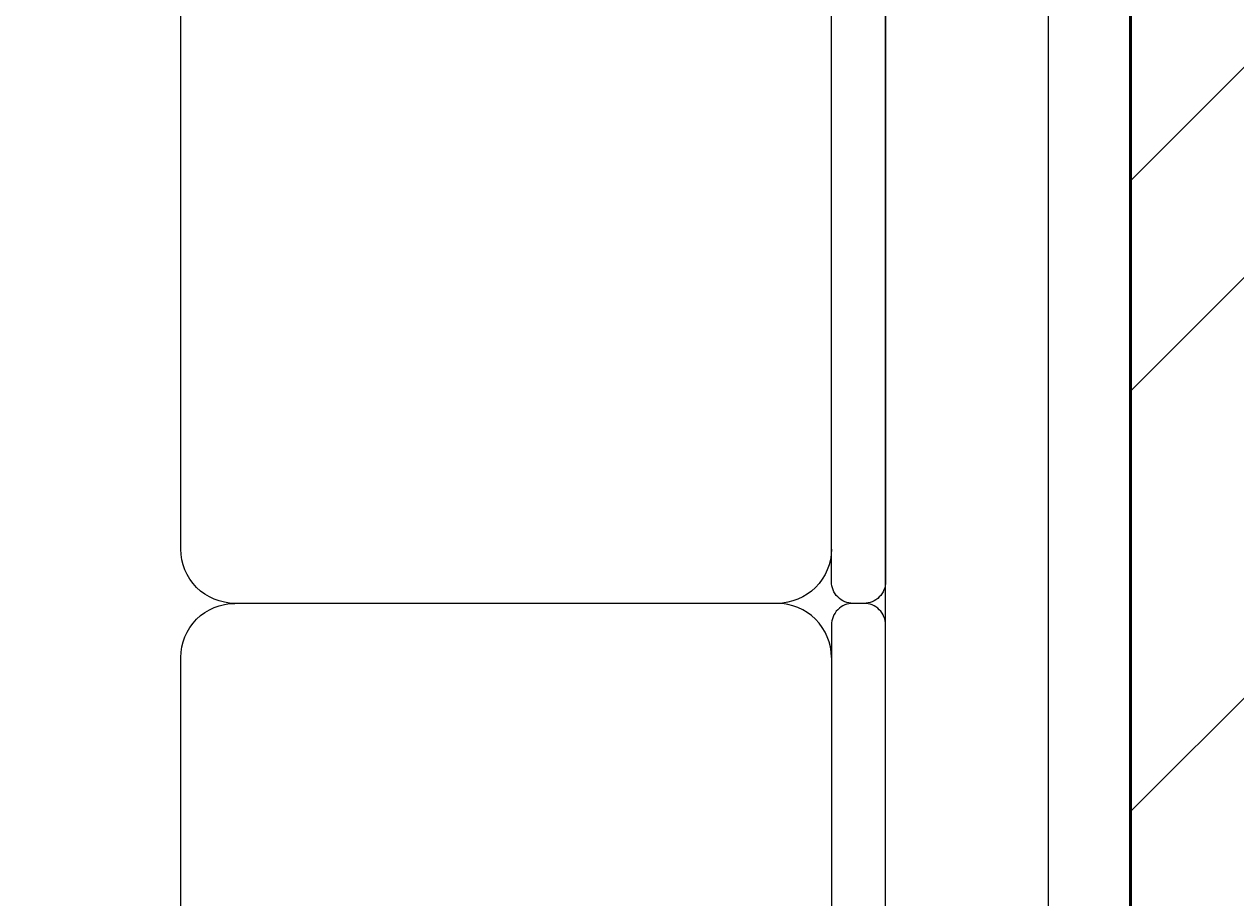
# Model space of a CAD drawing. Units: inches. Extents: x 963 to 2075, y 289 to 2657.
# Tile 23 of 98: x 1485 to 1511, y 1763 to 1781. Entities that reach past the tile are written whole.
import ezdxf

# ---------------------------------------------------------------- set-up
doc = ezdxf.new("R2010")
doc.units = ezdxf.units.IN
for name, color, linetype, lineweight in [('A-ANNO-DIMS', 2, 'Continuous', 18), ('A-FURN', 8, 'Continuous', 18), ('A-WALL', 7, 'Continuous', 50), ('A-WALL-PATT', 8, 'Continuous', 13)]:
    doc.layers.add(name, color=color, linetype=linetype, lineweight=lineweight)
doc.styles.get("Standard").update_dxf_attribs({"font": 'arial.ttf'})
doc.dimstyles.get("Standard").update_dxf_attribs({"dimtxt": 0.18, "dimasz": 0.18, "dimexe": 0.18, "dimexo": 0.0625, "dimgap": 0.09, "dimtad": 0, "dimtih": 1, "dimtoh": 1, "dimdec": 4, "dimzin": 0, "dimdsep": 46, "dimtxsty": 'Standard', "dimcen": 0.09, "dimadec": 0, "dimazin": 0, "dimtfac": 1, "dimtdec": 4, "dimtofl": 0, "dimtmove": 0, "dimatfit": 3, "dimfxl": 1, "dimtolj": 1, "dimtzin": 0, "dimarcsym": 0})

# ---------------------------------------------------------------- blocks, each defined once
blk = doc.blocks.new('SOFA-3SEAT')
at = {"ltscale": 0.03}
blk.add_lwpolyline([(2.442, 16.426, -0.414214), (0.124, 18.743), (0.124, 32.649, -0.414214), (1.283, 33.808, -0.414214), (0.124, 34.967), (0.124, 46.555, -0.414214), (1.283, 47.713, -0.414214), (0.124, 48.872), (0.124, 62.778, -0.414214), (2.442, 65.095), (16.347, 65.095, -0.414214), (18.665, 62.778), (18.665, 18.743, -0.414214), (16.347, 16.426)], format="xyb", close=True, dxfattribs=at)
blk.add_lwpolyline([(15.189, 24.268), (15.189, 51.011)])
blk.add_lwpolyline([(15.189, 47.25), (15.189, 34.271, -0.414214), (14.725, 33.808), (14.493, 33.808, -0.414214), (14.03, 34.271), (14.03, 47.25, -0.414214), (14.493, 47.713), (14.725, 47.713, -0.414214)], format="xyb", close=True)
for points in [[(14.03, 34.967, -0.414214), (12.871, 33.808)], [(14.03, 32.649, 0.414214), (12.871, 33.808), (1.283, 33.808, 0.414214)], [(15.189, 24.268), (15.189, 33.344, 0.414214), (14.725, 33.808), (14.493, 33.808, 0.414214), (14.03, 33.344), (14.03, 25.435, 0.414214)]]:
    blk.add_lwpolyline(points, format="xyb")
blk = doc.blocks.new('*D28')
at = {"layer": 'A-ANNO-DIMS', "color": 0, "lineweight": -2, "transparency": 16777216}
for p, q in [((1506.727, 1816.319), (1519.012, 1816.319)), ((1518.832, 1816.139), (1518.832, 1775.944)), ((1518.832, 1735.382), (1518.832, 1775.577)), ((1506.727, 1735.202), (1519.012, 1735.202))]:
    blk.add_line(p, q, dxfattribs=at)
at = {"layer": 'A-ANNO-DIMS', "color": 0, "transparency": 16777216}
for points in [[(1518.802, 1816.139), (1518.862, 1816.139), (1518.832, 1816.319)], [(1518.802, 1735.382), (1518.862, 1735.382), (1518.832, 1735.202)]]:
    blk.add_solid(points, dxfattribs=at)
at = {"layer": 'Defpoints', "color": 0, "transparency": 16777216}
for p in [(1506.665, 1816.319), (1518.832, 1816.319), (1506.665, 1735.202)]:
    blk.add_point(p, dxfattribs=at)
at = {"layer": 'A-ANNO-DIMS', "color": 0, "transparency": 16777216, "insert": (1518.832, 1775.761), "char_height": 0.18, "attachment_point": 5}
blk.add_mtext('\\A1;3-SEAT SOFA 81 TYP.', dxfattribs=at)

msp = doc.modelspace()

# ---------------------------------------------------------------- hatches: boundary and pattern name
at = {"layer": 'A-WALL-PATT'}
h = msp.add_hatch(dxfattribs=at)
h.set_pattern_fill('ANSI32', color=256)
h.paths.add_polyline_path([(1473.609, 2163.068), (1473.609, 2165.318), (1376.422, 2165.318), (1376.422, 2227.983), (1371.922, 2227.983), (1371.922, 2214.818), (1368.405, 2214.818), (1368.405, 2210.318), (1371.922, 2210.318), (1371.922, 2160.818), (1395.922, 2160.818), (1395.922, 2090.318), (1217.345, 2090.318), (1217.345, 2085.818), (1395.922, 2085.818), (1458.922, 2085.818), (1458.922, 2108.318), (1454.422, 2108.318), (1454.422, 2090.318), (1400.422, 2090.318), (1400.422, 2160.818), (1473.609, 2160.818)])
h.paths.add_polyline_path([(1649.422, 2210.318), (1653.225, 2210.318), (1653.225, 2214.818), (1649.422, 2214.818), (1649.422, 2227.983), (1644.922, 2227.983), (1644.922, 2165.318), (1550.099, 2165.318), (1550.099, 2160.818), (1620.922, 2160.818), (1620.922, 2112.818), (1555.446, 2112.818), (1555.446, 2108.318), (1584.327, 2108.318), (1584.327, 2084.916), (1588.827, 2084.916), (1588.827, 2108.318), (1625.422, 2108.318), (1667.951, 2108.318), (1667.951, 2022.667), (1588.827, 2022.667), (1588.827, 2047.408), (1584.327, 2047.408), (1584.327, 1996.003), (1588.827, 1996.003), (1588.827, 2018.318), (1667.951, 2018.167), (1667.951, 1928.318), (1625.422, 1928.318), (1625.422, 1923.818), (1672.451, 1923.818), (1672.451, 1928.318), (1672.451, 1946.663), (1785.446, 1946.663), (1785.446, 1951.163), (1743.034, 1951.163), (1743.034, 2017.922), (1841.422, 2017.922), (1841.422, 2014.775), (1845.922, 2014.775), (1845.922, 2017.922), (1905.922, 2017.922), (1905.922, 1987.511), (1910.422, 1987.511), (1910.422, 2022.422), (1910.422, 2068.517), (1905.922, 2068.517), (1905.922, 2022.422), (1845.922, 2022.422), (1845.922, 2025.851), (1843.672, 2025.851), (1841.422, 2025.851), (1841.422, 2022.422), (1743.034, 2022.422), (1743.034, 2084.031), (1768.451, 2084.031), (1785.446, 2084.031), (1785.446, 2088.531), (1672.451, 2088.531), (1672.451, 2112.818), (1667.951, 2112.818), (1625.422, 2112.818), (1625.422, 2160.818), (1649.422, 2160.818)])
h.paths.add_polyline_path([(1672.451, 2084.031), (1738.534, 2084.031), (1738.534, 1951.163), (1672.451, 1951.163)], flags=16)
h.paths.add_polyline_path([(1672.451, 2084.031), (1738.534, 2084.031), (1705.492, 2017.597)], flags=0)
h.paths.add_polyline_path([(1262.766, 2085.818), (1258.266, 2085.818), (1258.266, 2023.278), (1184.422, 2023.278), (1184.422, 2018.778), (1258.266, 2018.778), (1258.266, 1950.818), (1262.766, 1950.818)])
h.paths.add_polyline_path([(1312.266, 2085.818), (1307.766, 2085.818), (1307.766, 1950.818), (1312.266, 1950.818)])
h.paths.add_polyline_path([(1458.922, 1950.818), (1395.922, 1950.818), (1216.568, 1950.818), (1216.568, 1946.318), (1346.422, 1946.318), (1395.922, 1946.318), (1395.922, 1875.818), (1371.922, 1875.818), (1371.922, 1826.318), (1368.931, 1826.318), (1368.931, 1821.818), (1371.922, 1821.818), (1371.922, 1813.622), (1376.422, 1813.622), (1376.422, 1871.318), (1474.504, 1871.318), (1474.504, 1873.568), (1474.504, 1875.818), (1400.422, 1875.818), (1400.422, 1946.318), (1454.422, 1946.318), (1454.422, 1928.318), (1458.922, 1928.318)])
h.paths.add_polyline_path([(1184.422, 2120.778), (1167.922, 2120.778), (1167.922, 2134.812), (1165.672, 2134.812), (1163.422, 2134.812), (1163.422, 2120.778), (1119.922, 2120.778), (1119.922, 2098.095), (1124.422, 2098.095), (1124.422, 2116.278), (1167.922, 2116.278), (1179.922, 2116.278), (1179.922, 2045.916), (1184.422, 2045.916), (1184.422, 2090.318), (1184.422, 2116.278)])
h.paths.add_polyline_path([(1124.422, 2018.778), (1179.922, 2018.778), (1179.922, 2016.294), (1184.422, 2016.294), (1184.422, 2023.278), (1184.422, 2026.588), (1182.172, 2026.588), (1179.922, 2026.588), (1179.922, 2023.278), (1124.422, 2023.278), (1124.422, 2074.095), (1119.922, 2074.095), (1119.922, 2018.778), (1119.922, 1979.633), (1124.422, 1979.633)])
h.paths.add_polyline_path([(1184.422, 1925.778), (1184.422, 1946.318), (1184.422, 1996.073), (1182.172, 1996.073), (1179.922, 1996.073), (1179.922, 1925.778), (1124.422, 1925.778), (1124.422, 1955.633), (1119.922, 1955.502), (1119.922, 1921.278), (1158.922, 1921.278), (1158.922, 1909.983), (1163.422, 1909.983), (1163.422, 1921.278), (1184.422, 1921.278)])
h.paths.add_polyline_path([(1341.449, 1826.318), (1163.422, 1826.318), (1163.422, 1849.983), (1158.922, 1849.983), (1158.922, 1821.818), (1158.922, 1804.033), (1163.422, 1804.033), (1163.422, 1821.818), (1341.449, 1821.818)])
h.paths.add_polyline_path([(1222.981, 1713.818), (1163.422, 1713.818), (1163.422, 1744.033), (1161.172, 1744.033), (1158.922, 1744.033), (1158.922, 1713.818), (1119.922, 1713.818), (1119.922, 1694.65), (1124.422, 1694.65), (1124.422, 1709.318), (1158.922, 1709.318), (1222.981, 1709.318)])
h.paths.add_polyline_path([(1328.422, 1713.818), (1252.042, 1713.818), (1252.042, 1711.568), (1252.042, 1709.318), (1256.422, 1709.318), (1256.422, 1547.318), (1232.937, 1547.318), (1232.937, 1545.068), (1232.937, 1542.818), (1292.422, 1542.818), (1292.422, 1527.634), (1296.922, 1527.634), (1296.922, 1542.818), (1299.464, 1542.818), (1299.464, 1547.318), (1260.922, 1547.318), (1260.922, 1658.318), (1343.661, 1658.318), (1343.661, 1660.568), (1343.661, 1662.818), (1328.422, 1662.818), (1328.422, 1676.589), (1327.402, 1676.589), (1323.922, 1676.589), (1323.922, 1662.818), (1260.922, 1662.818), (1260.922, 1709.318), (1323.922, 1709.318), (1323.922, 1699.851), (1328.422, 1699.851)])
h.paths.add_polyline_path([(1649.422, 1875.818), (1625.422, 1875.818), (1625.422, 1928.318), (1620.922, 1928.318), (1588.827, 1928.318), (1588.827, 1950.59), (1584.327, 1950.59), (1584.327, 1928.318), (1555.446, 1928.318), (1555.446, 1923.818), (1620.922, 1923.818), (1620.922, 1875.818), (1548.952, 1875.818), (1548.952, 1873.568), (1548.952, 1871.318), (1644.922, 1871.318), (1644.922, 1813.622), (1649.422, 1813.622), (1649.422, 1821.818), (1652.045, 1821.818), (1652.045, 1824.068), (1652.045, 1826.318), (1649.422, 1826.318)])
h.paths.add_polyline_path([(1512.922, 1871.318), (1516.476, 1871.318), (1516.476, 1875.818), (1512.922, 1875.818), (1512.922, 1923.818), (1512.922, 1928.318), (1512.922, 1930.827), (1508.422, 1930.827), (1508.422, 1875.818), (1504.411, 1875.818), (1504.411, 1871.318), (1508.422, 1871.318), (1508.422, 1713.818), (1376.422, 1713.818), (1376.422, 1743.325), (1371.922, 1743.325), (1371.922, 1709.318), (1371.922, 1706.01), (1376.422, 1706.01), (1376.422, 1709.318), (1508.422, 1709.318), (1508.422, 1547.318), (1501.871, 1547.318), (1501.871, 1542.818), (1508.422, 1542.818), (1508.422, 1482.818), (1508.422, 1436.318), (1512.922, 1436.318), (1512.922, 1542.818), (1519.318, 1542.818), (1519.318, 1545.068), (1519.318, 1547.318), (1512.922, 1547.318), (1512.922, 1709.318), (1644.922, 1709.318), (1644.922, 1707.548), (1649.422, 1707.548), (1649.422, 1709.318), (1649.422, 1743.325), (1644.922, 1743.325), (1644.922, 1713.818), (1512.922, 1713.818)])
h.paths.add_polyline_path([(1129.884, 1545.068), (1129.884, 1547.318), (1124.422, 1547.318), (1095.922, 1547.318), (1095.922, 1614.818), (1124.422, 1614.818), (1124.422, 1619.318), (1095.922, 1619.318), (1091.422, 1619.318), (1091.422, 1542.818), (1095.922, 1542.818), (1119.922, 1542.818), (1129.884, 1542.818)])
h.paths.add_polyline_path([(1208.422, 1542.818), (1211.74, 1542.818), (1211.74, 1547.318), (1198.851, 1547.318), (1198.851, 1542.818), (1203.922, 1542.818), (1203.922, 1478.318), (1208.422, 1478.318), (1296.922, 1478.318), (1296.922, 1503.634), (1292.422, 1503.634), (1292.422, 1482.818), (1208.422, 1482.818)])
h.paths.add_polyline_path([(1430.422, 1542.818), (1435.699, 1542.818), (1435.699, 1545.068), (1435.699, 1547.318), (1422.658, 1547.318), (1422.658, 1545.068), (1422.658, 1542.818), (1425.922, 1542.818), (1425.922, 1482.857), (1341.922, 1482.857), (1341.922, 1502.732), (1337.422, 1502.732), (1337.422, 1478.357), (1425.922, 1478.357), (1425.922, 1440.818), (1425.922, 1436.318), (1430.422, 1436.318)])
h.paths.add_polyline_path([(1698.482, 2004.259), (1727.695, 2004.259), (1727.695, 2022.916), (1698.482, 2022.916)], flags=8)

# ---------------------------------------------------------------- linework, layer by layer
at = {"layer": 'A-WALL'}
msp.add_line((1508.422, 1871.318), (1508.422, 1713.818), dxfattribs=at)

# ---------------------------------------------------------------- block references
at = {"layer": 'A-FURN'}
msp.add_blockref('SOFA-3SEAT', (1488, 1735), dxfattribs=at)

# ---------------------------------------------------------------- dimensions: what is measured, and where the dimension line sits
at = {"layer": 'A-ANNO-DIMS'}
dim = msp.add_linear_dim(base=(1518.832, 1816.319), p1=(1506.665, 1735.202), p2=(1506.665, 1816.319), angle=90, text='3-SEAT SOFA <> TYP.', dimstyle='Standard', override={"dimdec": 0, "dimlfac": 1, "dimrnd": 0, "dimzin": 0, "dimdsep": 46, "dimlunit": 2}, dxfattribs=at)
dim.commit()
dim.dimension.update_dxf_attribs({"geometry": '*D28', "text_midpoint": (1518.832, 1775.761)})

doc.saveas('drawing.dxf')
